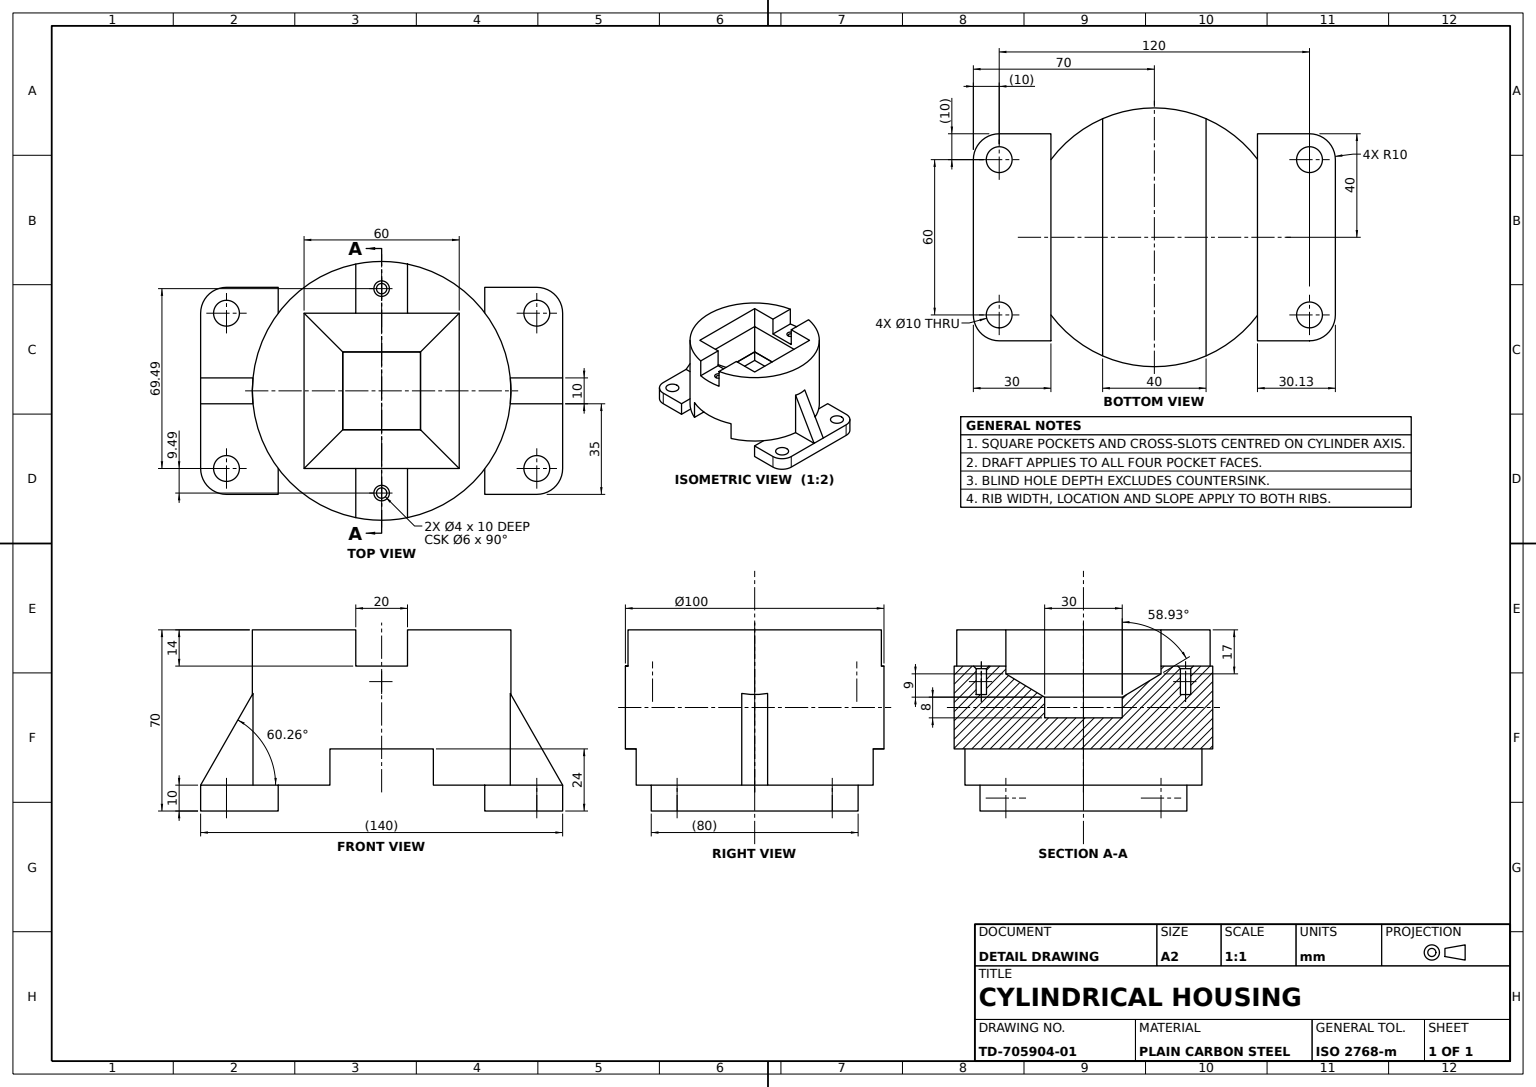
SolidWorks part; units mm, degrees
material "Plain Carbon Steel"
ref_plane "Front Plane" through (0, 0, 0) normal (0, 0, 1) x (1, 0, 0)
ref_plane "Top Plane" through (0, 0, 0) normal (0, 1, 0) x (1, 0, 0)
ref_plane "Right Plane" through (0, 0, 0) normal (1, 0, 0) x (0, 0, -1)
sketch "Base Plate Sketch" plane through (0, 0, 0) normal (0, 1, 0) x (1, 0, 0)
  line L0 (0, -40) -> (-60, -40)
  line L1 (70, 0) -> (70, 30)
  line L2 (60, 40) -> (-60, 40)
  line L3 (-70, 30) -> (-70, -30)
  line L4 (-60, -40) -> (60, -40)
  line L5 (70, -30) -> (70, 0)
  circle A0 centre (-60, -30) radius 5
  circle A1 centre (-60, 30) radius 5
  circle A2 centre (60, -30) radius 5
  circle A3 centre (60, 30) radius 5
  arc A4 (60, -40) -> (70, -30) centre (60, -30) ccw
  arc A5 (70, 30) -> (60, 40) centre (60, 30) ccw
  arc A6 (-70, -30) -> (-60, -40) centre (-60, -30) ccw
  arc A7 (-60, 40) -> (-70, 30) centre (-60, 30) ccw
  dimension "D1" = 10
  dimension "D2" = 10
  dimension "D3" = 10
  dimension "D4" = 10
  dimension "D9" = 67.082
  dimension "D10" = 60
  dimension "D11" = 60
  dimension "D12" = 67.082
  dimension "D13" = 60
  dimension "D14" = 67.082
  dimension "D15" = 60
  dimension "D16" = 67.082
  dimension "D17" = 10
  dimension "D18" = 67.082
  dimension "D19" = 60
  dimension "D5" = 120
  dimension "D6" = 60
  dimension "D7" = 60
  dimension "D8" = 30
extrude "Base Plate" add sketch "Base Plate Sketch" along normal blind 10 contours L2 A7 L3 A6 L0 L4 A4 L5 L1 A5 A0 A1 A2 A3
sketch "Body Cylinder Sketch" plane through (0, 10, 0) normal (0, 1, 0) x (1, 0, 0)
  circle A0 centre (0, 0) radius 50
  dimension "D1" = 100
extrude "Cylindrical Body Ø100" add sketch "Body Cylinder Sketch" along normal blind 60
sketch "Square Pocket Sketch" plane through (0, 70, 0) normal (0, 1, 0) x (1, 0, 0)
  line L1 (30, 0) -> (30, 30)
  line L2 (30, 30) -> (-30, 30)
  line L3 (-30, 30) -> (-30, -30)
  line L4 (-30, -30) -> (30, -30)
  line L5 (30, -30) -> (30, 0)
  dimension "D1" = 60
  dimension "D2" = 60
  dimension "D3" = 30
  dimension "D4" = 30
  dimension "D5" = 30
extrude "Square Pocket 60x60" cut sketch "Square Pocket Sketch" against normal blind 17
sketch "Lower Pocket Sketch" plane through (0, 53, 0) normal (0, 1, 0) x (1, 0, 0)
  line L9 (30, -30) -> (30, 30) construction
  line L10 (15, 0) -> (15, 15)
  line L11 (15, 15) -> (-15, 15)
  line L12 (-15, 15) -> (-15, -15)
  line L13 (-15, -15) -> (15, -15)
  line L14 (15, -15) -> (15, 0)
  line L15 (30, 30) -> (-30, 30) construction
  dimension "D1" = 15
  dimension "D2" = 45
  dimension "D3" = 15
extrude "Lower Pocket" cut sketch "Lower Pocket Sketch" against normal blind 17
ref_plane "Offset Plane 15mm" through (0, 0, 15) normal (0, 0, 1) x (1, 0, 0)
sketch "Drafted Boss Sketch" plane through (0, 53, 0) normal (0, 1, 0) x (1, 0, 0)
  line L0 (-15, 15) -> (15, 15)
  line L1 (15, 15) -> (15, -15)
  line L2 (15, -15) -> (-15, -15)
  line L3 (-15, -15) -> (-15, 15)
extrude "Drafted Boss" add sketch "Drafted Boss Sketch" along normal blind 9 draft 58.93 separate body draft outward yes
sketch "Slot A Sketch" plane through (0, 62, 0) normal (0, 1, 0) x (1, 0, 0)
  line L0 (-29.9371, 29.9371) -> (-29.9371, -29.9371) construction
  line L1 (15, 0) -> (15, 15)
  line L2 (15, 15) -> (-15, 15)
  line L3 (-15, 15) -> (-15, -15)
  line L4 (-15, -15) -> (15, -15)
  line L5 (15, -15) -> (15, 0)
  dimension "D1" = 14.9371
  dimension "D2" = 44.9371
  dimension "D3" = 14.9371
extrude "Slot A" cut sketch "Slot A Sketch" against normal blind 34
sketch "Inner Boss Sketch" plane through (0, 70, 0) normal (0, 1, 0) x (1, 0, 0)
  line L0 (-30, 30) -> (30, 30)
  line L1 (30, 30) -> (30, -30)
  line L2 (30, -30) -> (-30, -30)
  line L3 (-30, -30) -> (-30, 30)
extrude "Inner Boss" add sketch "Inner Boss Sketch" against normal blind 44
sketch "Slot B Sketch" plane through (0, 70, 0) normal (0, 1, 0) x (1, 0, 0)
  line L1 (15, 0) -> (15, 15)
  line L2 (15, 15) -> (-15, 15)
  line L3 (-15, 15) -> (-15, -15)
  line L4 (-15, -15) -> (15, -15)
  line L5 (15, -15) -> (15, 0)
  circle A0 centre (0, 0) radius 50 construction
  dimension "D1" = 15
  dimension "D2" = 15
  dimension "D3" = 15
extrude "Slot B" cut sketch "Slot B Sketch" against normal blind 34
sketch "Channel Sketch" plane through (0, 70, 0) normal (0, 1, 0) x (1, 0, 0)
  line L0 (-15, 15) -> (-15, -15) construction
  line L1 (30, 0) -> (30, 30)
  line L2 (30, 30) -> (-30, 30)
  line L3 (-30, 30) -> (-30, -30)
  line L4 (-30, -30) -> (30, -30)
  line L5 (30, -30) -> (30, 0)
  line L6 (-15, -15) -> (15, -15) construction
  dimension "D1" = 45
  dimension "D2" = 15
  dimension "D3" = 15
extrude "Channel Cut" cut sketch "Channel Sketch" against normal blind 17
sketch "Drafted Channel Sketch" plane through (0, 53, 0) normal (0, 1, 0) x (1, 0, 0)
  line L0 (-30, 30) -> (30, 30)
  line L1 (30, 30) -> (30, -30)
  line L2 (30, -30) -> (-30, -30)
  line L3 (-30, -30) -> (-30, 30)
extrude "Drafted Channel Cut" cut sketch "Drafted Channel Sketch" against normal blind 9 draft 58.93
sketch "Step Pocket Sketch" plane through (0, 70, 0) normal (0, 1, 0) x (1, 0, 0)
  line L0 (10, -30) -> (10, -50)
  line L1 (30, 30) -> (-30, 30) construction
  line L2 (0, 30) -> (10, 30)
  line L3 (30, 30) -> (-30, 30) construction
  line L4 (10, 30) -> (10, 50)
  line L5 (10, 50) -> (-10, 50)
  line L6 (-10, 50) -> (-10, 30)
  line L7 (-10, 30) -> (0, 30)
  line L8 (-30, -30) -> (30, -30) construction
  line L9 (10, -50) -> (-10, -50)
  line L10 (-10, -50) -> (-10, -30)
  line L11 (-30, -30) -> (30, -30) construction
  line L12 (-10, -30) -> (10, -30)
  line L13 (-30, 30) -> (-30, -30) construction
  dimension "D1" = 20
extrude "Step Pocket" cut sketch "Step Pocket Sketch" against normal blind 14
sketch "Pad Hole Chamfer Sketch" plane through (0, 56, 0) normal (0, 1, 0) x (1, 0, 0)
  line L0 (-10, 48.9898) -> (-10, 30) construction
  circle A0 centre (0, -39.4949) radius 3
  circle A1 centre (0, 39.4949) radius 3
  dimension "D1" = 6
  dimension "D2" = 10
  dimension "D3" = 9.4949
  dimension "D4" = 69.4949
extrude "Pad Hole Chamfer" cut sketch "Pad Hole Chamfer Sketch" against normal blind 1 draft 45
sketch "Pad Hole Sketch" plane through (0, 55, 0) normal (0, 1, 0) x (1, 0, 0)
  circle A0 centre (0, 39.4949) radius 2
  circle A1 centre (0, -39.4949) radius 2
  dimension "D1" = 4
extrude "Pad Hole" cut sketch "Pad Hole Sketch" against normal blind 10
sketch "Left Rib Sketch" plane through (0, 0, 0) normal (0, 0, 1) x (1, 0, 0)
  line L1 (-50, 45) -> (-70, 10)
  dimension "D1" = 20
  dimension "D2" = 35
rib "Left Support Rib" sketch "Left Rib Sketch" sketch "Left Rib Sketch" thickness 10 extrusion direction parallel to sketch draft on no parameters "D1"=10
sketch "Right Rib Sketch" plane through (0, 0, 0) normal (0, 0, 1) x (1, 0, 0)
  line L1 (50, 10) -> (50, 70) construction
  line L2 (50, 45) -> (70, 10)
  dimension "D1" = 35
rib "Right Support Rib" sketch "Right Rib Sketch" sketch "Right Rib Sketch" thickness 10 extrusion direction parallel to sketch draft on no parameters "D1"=10
ref_plane "Side Cut Plane" through (0, 0, 50) normal (0, 0, 1) x (1, 0, 0)
sketch "Side Cut A Sketch" plane through (0, 0, 50) normal (0, 0, 1) x (1, 0, 0)
  line L0 (0, 10) -> (-40, 10)
  line L1 (-30, 10) -> (30, 10) construction
  line L2 (-30, 10) -> (-60, 10) construction
  line L3 (-40, 10) -> (-40, 0)
  line L4 (60, 0) -> (-60, 0) construction
  line L5 (-40, 0) -> (39.8747, 0)
  line L6 (39.8747, 0) -> (39.8747, 10)
  line L7 (49.7494, 10) -> (30, 10) construction
  line L8 (0, 10) -> (39.8747, 10)
  dimension "D1" = 40
extrude "Side Cut A" cut sketch "Side Cut A Sketch" against normal blind 126
sketch "Side Cut B Sketch" plane through (0, 0, 50) normal (0, 0, 1) x (1, 0, 0)
  line L0 (0, 0) -> (20, 0)
  line L1 (20, 0) -> (20, 24)
  line L2 (20, 24) -> (-20, 24)
  line L3 (-20, 24) -> (-20, 0)
  line L4 (-20, 0) -> (0, 0)
  dimension "D1" = 20
  dimension "D2" = 24
extrude "Side Cut B" cut sketch "Side Cut B Sketch" against normal blind 202
